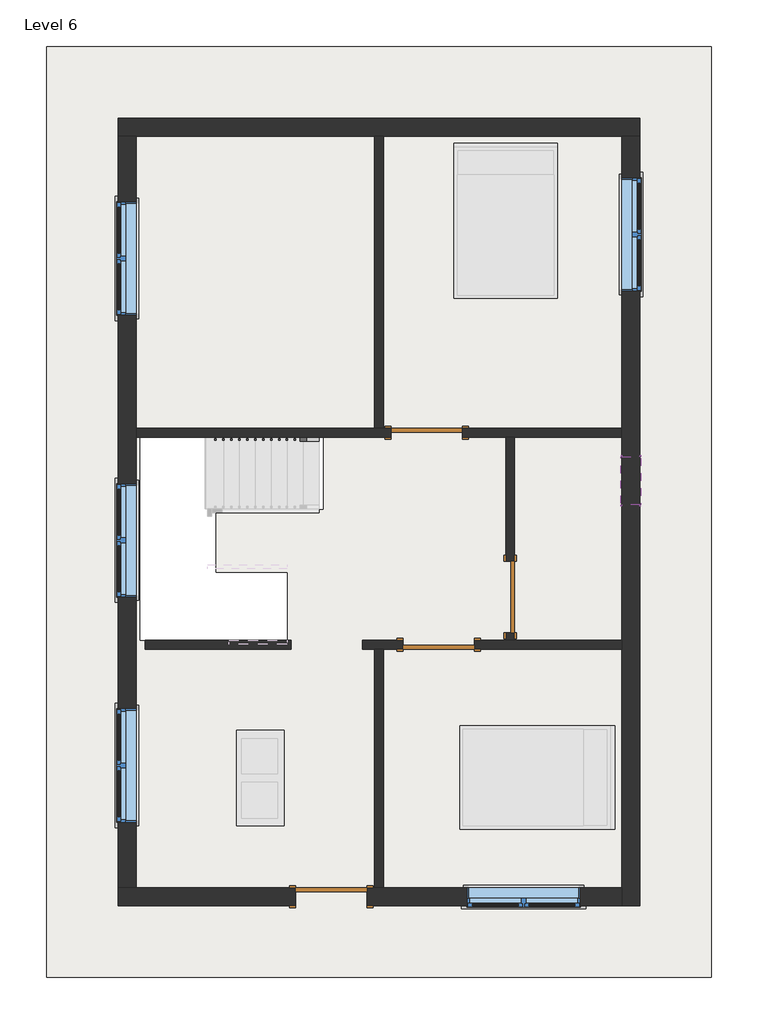
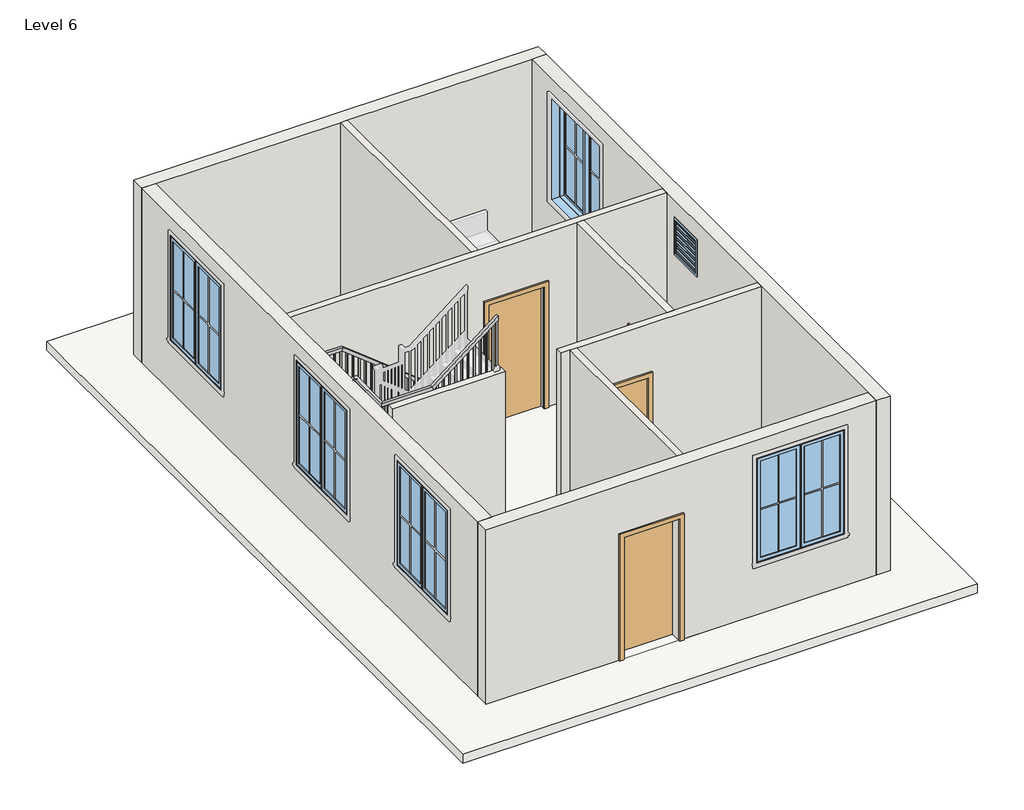
# One storey, part 1 of 2: 10 walls, 6 windows, 4 doors, 1 railing, 1 roof, 1 slab.
"""IFC4 building model written with IfcOpenShell, lengths in millimetres."""

from ifc_helpers import new_model, si_unit, frame, origin, place, context, project, spatial, polyline, outline, extrude, faceted_brep, transform, mapped, element, save
from components import door_e5f9f3c4, door_0ca8825f, window_9ac97e1a, window_f2d8fef0

model = new_model("IFC4")

# Units and contexts
model_context = context("Model", 3, world=origin())
ifc_project = project(units=[si_unit("LENGTHUNIT", "METRE", prefix="MILLI")], contexts=[model_context])

# Site, building, storey
site = spatial("IfcSite", under=ifc_project)
building = spatial("IfcBuilding", under=site)
storey = spatial("IfcBuildingStorey", under=building, Name="Level 6", Elevation=12801.6)

# Doors
placement = place(None, origin())
door_shape = door_e5f9f3c4(model_context)
element("IfcDoor", 1, ObjectType="Single-Flush : 36\" x 84\"", at=placement, inside=storey, context=model_context, shape_type="MappedRepresentation", body=[
    mapped(door_shape, transform((-2225.1840247, 979.1819954, 12801.6), x_axis=(1.0, 0.0, 0.0), y_axis=(0.0, 1.0, 0.0), z_axis=(0.0, 0.0, 1.0))),
])
element("IfcDoor", 2, ObjectType="Single-Flush : 36\" x 84\"", at=placement, inside=storey, context=model_context, shape_type="MappedRepresentation", body=[
    mapped(door_shape, transform((-1158.3840247, -1116.3180046, 12801.6), x_axis=(0.0, -1.0, 0.0), y_axis=(1.0, 0.0, 0.0), z_axis=(0.0, 0.0, 1.0))),
])
element("IfcDoor", 3, ObjectType="Single-Flush : 36\" x 84\"", at=placement, inside=storey, context=model_context, shape_type="MappedRepresentation", body=[
    mapped(door_shape, transform((-2072.7840247, -1725.9180046, 12801.6), x_axis=(-1.0, 0.0, 0.0), y_axis=(0.0, -1.0, 0.0), z_axis=(0.0, 0.0, 1.0))),
])
door_2_shape = door_0ca8825f(model_context)
element("IfcDoor", 4, ObjectType="Single-Flush : 36\" x 84\"", at=placement, inside=storey, context=model_context, shape_type="MappedRepresentation", body=[
    mapped(door_2_shape, transform((-3444.3840247, -4945.3680046, 12801.6), x_axis=(1.0, 0.0, 0.0), y_axis=(0.0, 1.0, 0.0), z_axis=(0.0, 0.0, 1.0))),
])

# Railing
element("IfcRailing", 5, ObjectType="Handrail - Rectangular", at=placement, inside=storey, context=model_context, shape_type="SolidModel", body=[
    faceted_brep([(-3603.1340247, 871.2319954, 13876.4210526), (-3603.1340247, 871.2319954, 13811.6980109), (-3603.1340247, 922.0319954, 13811.6980109), (-3603.1340247, 922.0319954, 13876.4210526), (-5097.5006913, 871.2319954, 15056.1842105), (-5115.1365442, 871.2319954, 15005.3842105), (-5115.1365442, 922.0319954, 15005.3842105), (-5097.5006913, 922.0319954, 15056.1842105), (-5889.1340247, 871.2319954, 15056.1842105), (-5889.1340247, 871.2319954, 15005.3842105), (-5939.9340247, 922.0319954, 15005.3842105), (-5939.9340247, 922.0319954, 15056.1842105), (-5889.1340247, 130.6632454, 15056.1842105), (-5889.1340247, 112.1228815, 15005.3842105), (-5939.9340247, 112.1228815, 15005.3842105), (-5939.9340247, 130.6632454, 15056.1842105), (-5889.1340247, -877.3992546, 15905.0789474), (-5889.1340247, -895.9396185, 15854.2789474), (-5939.9340247, -895.9396185, 15854.2789474), (-5939.9340247, -877.3992546, 15905.0789474), (-5889.1340247, -1617.9680046, 15905.0789474), (-5889.1340247, -1617.9680046, 15854.2789474), (-5939.9340247, -1668.7680046, 15854.2789474), (-5939.9340247, -1668.7680046, 15905.0789474), (-5097.5006913, -1617.9680046, 15905.0789474), (-5079.8648385, -1617.9680046, 15854.2789474), (-5079.8648385, -1668.7680046, 15854.2789474), (-5097.5006913, -1668.7680046, 15905.0789474), (-4009.5340247, -1617.9680046, 16764.0), (-4009.5340247, -1668.7680046, 16764.0), (-4009.5340247, -1668.7680046, 16699.2769583), (-4009.5340247, -1617.9680046, 16699.2769583)], [[[0, 1, 2, 3]], [[1, 0, 4, 5]], [[2, 1, 5, 6]], [[3, 2, 6, 7]], [[0, 3, 7, 4]], [[5, 4, 8, 9]], [[6, 5, 9, 10]], [[7, 6, 10, 11]], [[4, 7, 11, 8]], [[9, 8, 12, 13]], [[10, 9, 13, 14]], [[11, 10, 14, 15]], [[8, 11, 15, 12]], [[13, 12, 16, 17]], [[14, 13, 17, 18]], [[15, 14, 18, 19]], [[12, 15, 19, 16]], [[17, 16, 20, 21]], [[18, 17, 21, 22]], [[19, 18, 22, 23]], [[16, 19, 23, 20]], [[21, 20, 24, 25]], [[22, 21, 25, 26]], [[23, 22, 26, 27]], [[20, 23, 27, 24]], [[28, 29, 30, 31]], [[25, 24, 28, 31]], [[26, 25, 31, 30]], [[27, 26, 30, 29]], [[24, 27, 29, 28]]]),
    extrude(outline(polyline([(16646.6388004, -4076.2090247), (16631.5993267, -4095.2590247), (15689.1789474, -4095.2590247), (15689.1789474, -4076.2090247), (16646.6388004, -4076.2090247)])), frame((0.0, -1652.8930046, 0.0), z_axis=(0.0, 1.0, 0.0), x_axis=(0.0, 0.0, 1.0)), (0.0, 0.0, 1.0), 19.05),
    extrude(outline(polyline([(16566.428274, -4177.8090247), (16551.3888004, -4196.8590247), (15689.1789474, -4196.8590247), (15689.1789474, -4177.8090247), (16566.428274, -4177.8090247)])), frame((0.0, -1652.8930046, 0.0), z_axis=(0.0, 1.0, 0.0), x_axis=(0.0, 0.0, 1.0)), (0.0, 0.0, 1.0), 19.05),
    extrude(outline(polyline([(16486.2177477, -4279.4090247), (16471.178274, -4298.4590247), (15528.7578947, -4298.4590247), (15528.7578947, -4279.4090247), (16486.2177477, -4279.4090247)])), frame((0.0, -1652.8930046, 0.0), z_axis=(0.0, 1.0, 0.0), x_axis=(0.0, 0.0, 1.0)), (0.0, 0.0, 1.0), 19.05),
    extrude(outline(polyline([(16406.0072214, -4381.0090247), (16390.9677477, -4400.0590247), (15528.7578947, -4400.0590247), (15528.7578947, -4381.0090247), (16406.0072214, -4381.0090247)])), frame((0.0, -1652.8930046, 0.0), z_axis=(0.0, 1.0, 0.0), x_axis=(0.0, 0.0, 1.0)), (0.0, 0.0, 1.0), 19.05),
    extrude(outline(polyline([(16325.7966951, -4482.6090247), (16310.7572214, -4501.6590247), (15368.3368421, -4501.6590247), (15368.3368421, -4482.6090247), (16325.7966951, -4482.6090247)])), frame((0.0, -1652.8930046, 0.0), z_axis=(0.0, 1.0, 0.0), x_axis=(0.0, 0.0, 1.0)), (0.0, 0.0, 1.0), 19.05),
    extrude(outline(polyline([(16245.5861688, -4584.2090247), (16230.5466951, -4603.2590247), (15368.3368421, -4603.2590247), (15368.3368421, -4584.2090247), (16245.5861688, -4584.2090247)])), frame((0.0, -1652.8930046, 0.0), z_axis=(0.0, 1.0, 0.0), x_axis=(0.0, 0.0, 1.0)), (0.0, 0.0, 1.0), 19.05),
    extrude(outline(polyline([(16165.3756425, -4685.8090247), (16150.3361688, -4704.8590247), (15207.9157895, -4704.8590247), (15207.9157895, -4685.8090247), (16165.3756425, -4685.8090247)])), frame((0.0, -1652.8930046, 0.0), z_axis=(0.0, 1.0, 0.0), x_axis=(0.0, 0.0, 1.0)), (0.0, 0.0, 1.0), 19.05),
    extrude(outline(polyline([(16085.1651161, -4787.4090247), (16070.1256425, -4806.4590247), (15207.9157895, -4806.4590247), (15207.9157895, -4787.4090247), (16085.1651161, -4787.4090247)])), frame((0.0, -1652.8930046, 0.0), z_axis=(0.0, 1.0, 0.0), x_axis=(0.0, 0.0, 1.0)), (0.0, 0.0, 1.0), 19.05),
    extrude(outline(polyline([(16004.9545898, -4889.0090247), (15989.9151161, -4908.0590247), (15047.4947368, -4908.0590247), (15047.4947368, -4889.0090247), (16004.9545898, -4889.0090247)])), frame((0.0, -1652.8930046, 0.0), z_axis=(0.0, 1.0, 0.0), x_axis=(0.0, 0.0, 1.0)), (0.0, 0.0, 1.0), 19.05),
    extrude(outline(polyline([(15924.7440635, -4990.6090247), (15909.7045898, -5009.6590247), (15047.4947368, -5009.6590247), (15047.4947368, -4990.6090247), (15924.7440635, -4990.6090247)])), frame((0.0, -1652.8930046, 0.0), z_axis=(0.0, 1.0, 0.0), x_axis=(0.0, 0.0, 1.0)), (0.0, 0.0, 1.0), 19.05),
    extrude(outline(polyline([(-5111.2590247, -1652.8930046), (-5111.2590247, -1633.8430046), (-5092.2090247, -1633.8430046), (-5092.2090247, -1652.8930046), (-5111.2590247, -1652.8930046)])), frame((0.0, 0.0, 14887.0736842), z_axis=(0.0, 0.0, 1.0), x_axis=(1.0, 0.0, 0.0)), (0.0, 0.0, 1.0), 967.2052632),
    extrude(outline(polyline([(-5212.8590247, -1652.8930046), (-5212.8590247, -1633.8430046), (-5193.8090247, -1633.8430046), (-5193.8090247, -1652.8930046), (-5212.8590247, -1652.8930046)])), frame((0.0, 0.0, 14887.0736842), z_axis=(0.0, 0.0, 1.0), x_axis=(1.0, 0.0, 0.0)), (0.0, 0.0, 1.0), 967.2052632),
    extrude(outline(polyline([(-5314.4590247, -1652.8930046), (-5314.4590247, -1633.8430046), (-5295.4090247, -1633.8430046), (-5295.4090247, -1652.8930046), (-5314.4590247, -1652.8930046)])), frame((0.0, 0.0, 14887.0736842), z_axis=(0.0, 0.0, 1.0), x_axis=(1.0, 0.0, 0.0)), (0.0, 0.0, 1.0), 967.2052632),
    extrude(outline(polyline([(-5416.0590247, -1652.8930046), (-5416.0590247, -1633.8430046), (-5397.0090247, -1633.8430046), (-5397.0090247, -1652.8930046), (-5416.0590247, -1652.8930046)])), frame((0.0, 0.0, 14887.0736842), z_axis=(0.0, 0.0, 1.0), x_axis=(1.0, 0.0, 0.0)), (0.0, 0.0, 1.0), 967.2052632),
    extrude(outline(polyline([(-5517.6590247, -1652.8930046), (-5517.6590247, -1633.8430046), (-5498.6090247, -1633.8430046), (-5498.6090247, -1652.8930046), (-5517.6590247, -1652.8930046)])), frame((0.0, 0.0, 14887.0736842), z_axis=(0.0, 0.0, 1.0), x_axis=(1.0, 0.0, 0.0)), (0.0, 0.0, 1.0), 967.2052632),
    extrude(outline(polyline([(-5619.2590247, -1652.8930046), (-5619.2590247, -1633.8430046), (-5600.2090247, -1633.8430046), (-5600.2090247, -1652.8930046), (-5619.2590247, -1652.8930046)])), frame((0.0, 0.0, 14887.0736842), z_axis=(0.0, 0.0, 1.0), x_axis=(1.0, 0.0, 0.0)), (0.0, 0.0, 1.0), 967.2052632),
    extrude(outline(polyline([(-5720.8590247, -1652.8930046), (-5720.8590247, -1633.8430046), (-5701.8090247, -1633.8430046), (-5701.8090247, -1652.8930046), (-5720.8590247, -1652.8930046)])), frame((0.0, 0.0, 14887.0736842), z_axis=(0.0, 0.0, 1.0), x_axis=(1.0, 0.0, 0.0)), (0.0, 0.0, 1.0), 967.2052632),
    extrude(outline(polyline([(-5822.4590247, -1652.8930046), (-5822.4590247, -1633.8430046), (-5803.4090247, -1633.8430046), (-5803.4090247, -1652.8930046), (-5822.4590247, -1652.8930046)])), frame((0.0, 0.0, 14887.0736842), z_axis=(0.0, 0.0, 1.0), x_axis=(1.0, 0.0, 0.0)), (0.0, 0.0, 1.0), 967.2052632),
    extrude(outline(polyline([(-5924.0590247, -1532.2430046), (-5905.0090247, -1532.2430046), (-5905.0090247, -1551.2930046), (-5924.0590247, -1551.2930046), (-5924.0590247, -1532.2430046)])), frame((0.0, 0.0, 14887.0736842), z_axis=(0.0, 0.0, 1.0), x_axis=(1.0, 0.0, 0.0)), (0.0, 0.0, 1.0), 967.2052632),
    extrude(outline(polyline([(-5924.0590247, -1430.6430046), (-5905.0090247, -1430.6430046), (-5905.0090247, -1449.6930046), (-5924.0590247, -1449.6930046), (-5924.0590247, -1430.6430046)])), frame((0.0, 0.0, 14887.0736842), z_axis=(0.0, 0.0, 1.0), x_axis=(1.0, 0.0, 0.0)), (0.0, 0.0, 1.0), 967.2052632),
    extrude(outline(polyline([(-5924.0590247, -1329.0430046), (-5905.0090247, -1329.0430046), (-5905.0090247, -1348.0930046), (-5924.0590247, -1348.0930046), (-5924.0590247, -1329.0430046)])), frame((0.0, 0.0, 14887.0736842), z_axis=(0.0, 0.0, 1.0), x_axis=(1.0, 0.0, 0.0)), (0.0, 0.0, 1.0), 967.2052632),
    extrude(outline(polyline([(-5924.0590247, -1227.4430046), (-5905.0090247, -1227.4430046), (-5905.0090247, -1246.4930046), (-5924.0590247, -1246.4930046), (-5924.0590247, -1227.4430046)])), frame((0.0, 0.0, 14887.0736842), z_axis=(0.0, 0.0, 1.0), x_axis=(1.0, 0.0, 0.0)), (0.0, 0.0, 1.0), 967.2052632),
    extrude(outline(polyline([(-5924.0590247, -1125.8430046), (-5905.0090247, -1125.8430046), (-5905.0090247, -1144.8930046), (-5924.0590247, -1144.8930046), (-5924.0590247, -1125.8430046)])), frame((0.0, 0.0, 14887.0736842), z_axis=(0.0, 0.0, 1.0), x_axis=(1.0, 0.0, 0.0)), (0.0, 0.0, 1.0), 967.2052632),
    extrude(outline(polyline([(-5924.0590247, -1024.2430046), (-5905.0090247, -1024.2430046), (-5905.0090247, -1043.2930046), (-5924.0590247, -1043.2930046), (-5924.0590247, -1024.2430046)])), frame((0.0, 0.0, 14887.0736842), z_axis=(0.0, 0.0, 1.0), x_axis=(1.0, 0.0, 0.0)), (0.0, 0.0, 1.0), 967.2052632),
    extrude(outline(polyline([(-5924.0590247, -922.6430046), (-5905.0090247, -922.6430046), (-5905.0090247, -941.6930046), (-5924.0590247, -941.6930046), (-5924.0590247, -922.6430046)])), frame((0.0, 0.0, 14887.0736842), z_axis=(0.0, 0.0, 1.0), x_axis=(1.0, 0.0, 0.0)), (0.0, 0.0, 1.0), 967.2052632),
    extrude(outline(polyline([(-840.0930046, 15807.2502199), (-821.0430046, 15791.2081146), (-821.0430046, 14887.0736842), (-840.0930046, 14887.0736842), (-840.0930046, 15807.2502199)])), frame((-5924.0590247, 0.0, 0.0), z_axis=(1.0, 0.0, 0.0), x_axis=(0.0, 1.0, 0.0)), (0.0, 0.0, 1.0), 19.05),
    extrude(outline(polyline([(-738.4930046, 15721.6923251), (-719.4430046, 15705.6502199), (-719.4430046, 14726.6526316), (-738.4930046, 14726.6526316), (-738.4930046, 15721.6923251)])), frame((-5924.0590247, 0.0, 0.0), z_axis=(1.0, 0.0, 0.0), x_axis=(0.0, 1.0, 0.0)), (0.0, 0.0, 1.0), 19.05),
    extrude(outline(polyline([(-636.8930046, 15636.1344304), (-617.8430046, 15620.0923251), (-617.8430046, 14726.6526316), (-636.8930046, 14726.6526316), (-636.8930046, 15636.1344304)])), frame((-5924.0590247, 0.0, 0.0), z_axis=(1.0, 0.0, 0.0), x_axis=(0.0, 1.0, 0.0)), (0.0, 0.0, 1.0), 19.05),
    extrude(outline(polyline([(-535.2930046, 15550.5765357), (-516.2430046, 15534.5344304), (-516.2430046, 14566.2315789), (-535.2930046, 14566.2315789), (-535.2930046, 15550.5765357)])), frame((-5924.0590247, 0.0, 0.0), z_axis=(1.0, 0.0, 0.0), x_axis=(0.0, 1.0, 0.0)), (0.0, 0.0, 1.0), 19.05),
    extrude(outline(polyline([(-433.6930046, 15465.0186409), (-414.6430046, 15448.9765357), (-414.6430046, 14566.2315789), (-433.6930046, 14566.2315789), (-433.6930046, 15465.0186409)])), frame((-5924.0590247, 0.0, 0.0), z_axis=(1.0, 0.0, 0.0), x_axis=(0.0, 1.0, 0.0)), (0.0, 0.0, 1.0), 19.05),
    extrude(outline(polyline([(-332.0930046, 15379.4607462), (-313.0430046, 15363.4186409), (-313.0430046, 14405.8105263), (-332.0930046, 14405.8105263), (-332.0930046, 15379.4607462)])), frame((-5924.0590247, 0.0, 0.0), z_axis=(1.0, 0.0, 0.0), x_axis=(0.0, 1.0, 0.0)), (0.0, 0.0, 1.0), 19.05),
    extrude(outline(polyline([(-230.4930046, 15293.9028514), (-211.4430046, 15277.8607462), (-211.4430046, 14405.8105263), (-230.4930046, 14405.8105263), (-230.4930046, 15293.9028514)])), frame((-5924.0590247, 0.0, 0.0), z_axis=(1.0, 0.0, 0.0), x_axis=(0.0, 1.0, 0.0)), (0.0, 0.0, 1.0), 19.05),
    extrude(outline(polyline([(-128.8930046, 15208.3449567), (-109.8430046, 15192.3028514), (-109.8430046, 14245.3894737), (-128.8930046, 14245.3894737), (-128.8930046, 15208.3449567)])), frame((-5924.0590247, 0.0, 0.0), z_axis=(1.0, 0.0, 0.0), x_axis=(0.0, 1.0, 0.0)), (0.0, 0.0, 1.0), 19.05),
    extrude(outline(polyline([(-27.2930046, 15122.787062), (-8.2430046, 15106.7449567), (-8.2430046, 14245.3894737), (-27.2930046, 14245.3894737), (-27.2930046, 15122.787062)])), frame((-5924.0590247, 0.0, 0.0), z_axis=(1.0, 0.0, 0.0), x_axis=(0.0, 1.0, 0.0)), (0.0, 0.0, 1.0), 19.05),
    extrude(outline(polyline([(74.3069954, 15037.2291672), (93.3569954, 15021.187062), (93.3569954, 14084.9684211), (74.3069954, 14084.9684211), (74.3069954, 15037.2291672)])), frame((-5924.0590247, 0.0, 0.0), z_axis=(1.0, 0.0, 0.0), x_axis=(0.0, 1.0, 0.0)), (0.0, 0.0, 1.0), 19.05),
    extrude(outline(polyline([(-5924.0590247, 194.9569954), (-5905.0090247, 194.9569954), (-5905.0090247, 175.9069954), (-5924.0590247, 175.9069954), (-5924.0590247, 194.9569954)])), frame((0.0, 0.0, 14084.9684211), z_axis=(0.0, 0.0, 1.0), x_axis=(1.0, 0.0, 0.0)), (0.0, 0.0, 1.0), 920.4157895),
    extrude(outline(polyline([(-5924.0590247, 296.5569954), (-5905.0090247, 296.5569954), (-5905.0090247, 277.5069954), (-5924.0590247, 277.5069954), (-5924.0590247, 296.5569954)])), frame((0.0, 0.0, 14084.9684211), z_axis=(0.0, 0.0, 1.0), x_axis=(1.0, 0.0, 0.0)), (0.0, 0.0, 1.0), 920.4157895),
    extrude(outline(polyline([(-5924.0590247, 398.1569954), (-5905.0090247, 398.1569954), (-5905.0090247, 379.1069954), (-5924.0590247, 379.1069954), (-5924.0590247, 398.1569954)])), frame((0.0, 0.0, 14084.9684211), z_axis=(0.0, 0.0, 1.0), x_axis=(1.0, 0.0, 0.0)), (0.0, 0.0, 1.0), 920.4157895),
    extrude(outline(polyline([(-5924.0590247, 499.7569954), (-5905.0090247, 499.7569954), (-5905.0090247, 480.7069954), (-5924.0590247, 480.7069954), (-5924.0590247, 499.7569954)])), frame((0.0, 0.0, 14084.9684211), z_axis=(0.0, 0.0, 1.0), x_axis=(1.0, 0.0, 0.0)), (0.0, 0.0, 1.0), 920.4157895),
    extrude(outline(polyline([(-5924.0590247, 601.3569954), (-5905.0090247, 601.3569954), (-5905.0090247, 582.3069954), (-5924.0590247, 582.3069954), (-5924.0590247, 601.3569954)])), frame((0.0, 0.0, 14084.9684211), z_axis=(0.0, 0.0, 1.0), x_axis=(1.0, 0.0, 0.0)), (0.0, 0.0, 1.0), 920.4157895),
    extrude(outline(polyline([(-5924.0590247, 702.9569954), (-5905.0090247, 702.9569954), (-5905.0090247, 683.9069954), (-5924.0590247, 683.9069954), (-5924.0590247, 702.9569954)])), frame((0.0, 0.0, 14084.9684211), z_axis=(0.0, 0.0, 1.0), x_axis=(1.0, 0.0, 0.0)), (0.0, 0.0, 1.0), 920.4157895),
    extrude(outline(polyline([(-5924.0590247, 804.5569954), (-5905.0090247, 804.5569954), (-5905.0090247, 785.5069954), (-5924.0590247, 785.5069954), (-5924.0590247, 804.5569954)])), frame((0.0, 0.0, 14084.9684211), z_axis=(0.0, 0.0, 1.0), x_axis=(1.0, 0.0, 0.0)), (0.0, 0.0, 1.0), 920.4157895),
    extrude(outline(polyline([(-5828.8090247, 906.1569954), (-5828.8090247, 887.1069954), (-5847.8590247, 887.1069954), (-5847.8590247, 906.1569954), (-5828.8090247, 906.1569954)])), frame((0.0, 0.0, 14084.9684211), z_axis=(0.0, 0.0, 1.0), x_axis=(1.0, 0.0, 0.0)), (0.0, 0.0, 1.0), 920.4157895),
    extrude(outline(polyline([(-5727.2090247, 906.1569954), (-5727.2090247, 887.1069954), (-5746.2590247, 887.1069954), (-5746.2590247, 906.1569954), (-5727.2090247, 906.1569954)])), frame((0.0, 0.0, 14084.9684211), z_axis=(0.0, 0.0, 1.0), x_axis=(1.0, 0.0, 0.0)), (0.0, 0.0, 1.0), 920.4157895),
    extrude(outline(polyline([(-5625.6090247, 906.1569954), (-5625.6090247, 887.1069954), (-5644.6590247, 887.1069954), (-5644.6590247, 906.1569954), (-5625.6090247, 906.1569954)])), frame((0.0, 0.0, 14084.9684211), z_axis=(0.0, 0.0, 1.0), x_axis=(1.0, 0.0, 0.0)), (0.0, 0.0, 1.0), 920.4157895),
    extrude(outline(polyline([(-5524.0090247, 906.1569954), (-5524.0090247, 887.1069954), (-5543.0590247, 887.1069954), (-5543.0590247, 906.1569954), (-5524.0090247, 906.1569954)])), frame((0.0, 0.0, 14084.9684211), z_axis=(0.0, 0.0, 1.0), x_axis=(1.0, 0.0, 0.0)), (0.0, 0.0, 1.0), 920.4157895),
    extrude(outline(polyline([(-5422.4090247, 906.1569954), (-5422.4090247, 887.1069954), (-5441.4590247, 887.1069954), (-5441.4590247, 906.1569954), (-5422.4090247, 906.1569954)])), frame((0.0, 0.0, 14084.9684211), z_axis=(0.0, 0.0, 1.0), x_axis=(1.0, 0.0, 0.0)), (0.0, 0.0, 1.0), 920.4157895),
    extrude(outline(polyline([(-5320.8090247, 906.1569954), (-5320.8090247, 887.1069954), (-5339.8590247, 887.1069954), (-5339.8590247, 906.1569954), (-5320.8090247, 906.1569954)])), frame((0.0, 0.0, 14084.9684211), z_axis=(0.0, 0.0, 1.0), x_axis=(1.0, 0.0, 0.0)), (0.0, 0.0, 1.0), 920.4157895),
    extrude(outline(polyline([(-5219.2090247, 906.1569954), (-5219.2090247, 887.1069954), (-5238.2590247, 887.1069954), (-5238.2590247, 906.1569954), (-5219.2090247, 906.1569954)])), frame((0.0, 0.0, 14084.9684211), z_axis=(0.0, 0.0, 1.0), x_axis=(1.0, 0.0, 0.0)), (0.0, 0.0, 1.0), 920.4157895),
    extrude(outline(polyline([(-5117.6090247, 906.1569954), (-5117.6090247, 887.1069954), (-5136.6590247, 887.1069954), (-5136.6590247, 906.1569954), (-5117.6090247, 906.1569954)])), frame((0.0, 0.0, 14084.9684211), z_axis=(0.0, 0.0, 1.0), x_axis=(1.0, 0.0, 0.0)), (0.0, 0.0, 1.0), 920.4157895),
    extrude(outline(polyline([(14927.1256425, -5016.0090247), (14942.1651161, -5035.0590247), (14084.9684211, -5035.0590247), (14084.9684211, -5016.0090247), (14927.1256425, -5016.0090247)])), frame((0.0, 887.1069954, 0.0), z_axis=(0.0, 1.0, 0.0), x_axis=(0.0, 0.0, 1.0)), (0.0, 0.0, 1.0), 19.05),
    extrude(outline(polyline([(14846.9151161, -4914.4090247), (14861.9545898, -4933.4590247), (13924.5473684, -4933.4590247), (13924.5473684, -4914.4090247), (14846.9151161, -4914.4090247)])), frame((0.0, 887.1069954, 0.0), z_axis=(0.0, 1.0, 0.0), x_axis=(0.0, 0.0, 1.0)), (0.0, 0.0, 1.0), 19.05),
    extrude(outline(polyline([(14766.7045898, -4812.8090247), (14781.7440635, -4831.8590247), (13924.5473684, -4831.8590247), (13924.5473684, -4812.8090247), (14766.7045898, -4812.8090247)])), frame((0.0, 887.1069954, 0.0), z_axis=(0.0, 1.0, 0.0), x_axis=(0.0, 0.0, 1.0)), (0.0, 0.0, 1.0), 19.05),
    extrude(outline(polyline([(14686.4940635, -4711.2090247), (14701.5335372, -4730.2590247), (13764.1263158, -4730.2590247), (13764.1263158, -4711.2090247), (14686.4940635, -4711.2090247)])), frame((0.0, 887.1069954, 0.0), z_axis=(0.0, 1.0, 0.0), x_axis=(0.0, 0.0, 1.0)), (0.0, 0.0, 1.0), 19.05),
    extrude(outline(polyline([(14606.2835372, -4609.6090247), (14621.3230109, -4628.6590247), (13764.1263158, -4628.6590247), (13764.1263158, -4609.6090247), (14606.2835372, -4609.6090247)])), frame((0.0, 887.1069954, 0.0), z_axis=(0.0, 1.0, 0.0), x_axis=(0.0, 0.0, 1.0)), (0.0, 0.0, 1.0), 19.05),
    extrude(outline(polyline([(14526.0730109, -4508.0090247), (14541.1124846, -4527.0590247), (13603.7052632, -4527.0590247), (13603.7052632, -4508.0090247), (14526.0730109, -4508.0090247)])), frame((0.0, 887.1069954, 0.0), z_axis=(0.0, 1.0, 0.0), x_axis=(0.0, 0.0, 1.0)), (0.0, 0.0, 1.0), 19.05),
    extrude(outline(polyline([(14445.8624846, -4406.4090247), (14460.9019583, -4425.4590247), (13603.7052632, -4425.4590247), (13603.7052632, -4406.4090247), (14445.8624846, -4406.4090247)])), frame((0.0, 887.1069954, 0.0), z_axis=(0.0, 1.0, 0.0), x_axis=(0.0, 0.0, 1.0)), (0.0, 0.0, 1.0), 19.05),
    extrude(outline(polyline([(14365.6519583, -4304.8090247), (14380.6914319, -4323.8590247), (13443.2842105, -4323.8590247), (13443.2842105, -4304.8090247), (14365.6519583, -4304.8090247)])), frame((0.0, 887.1069954, 0.0), z_axis=(0.0, 1.0, 0.0), x_axis=(0.0, 0.0, 1.0)), (0.0, 0.0, 1.0), 19.05),
    extrude(outline(polyline([(14285.4414319, -4203.2090247), (14300.4809056, -4222.2590247), (13443.2842105, -4222.2590247), (13443.2842105, -4203.2090247), (14285.4414319, -4203.2090247)])), frame((0.0, 887.1069954, 0.0), z_axis=(0.0, 1.0, 0.0), x_axis=(0.0, 0.0, 1.0)), (0.0, 0.0, 1.0), 19.05),
    extrude(outline(polyline([(14205.2309056, -4101.6090247), (14220.2703793, -4120.6590247), (13282.8631579, -4120.6590247), (13282.8631579, -4101.6090247), (14205.2309056, -4101.6090247)])), frame((0.0, 887.1069954, 0.0), z_axis=(0.0, 1.0, 0.0), x_axis=(0.0, 0.0, 1.0)), (0.0, 0.0, 1.0), 19.05),
    extrude(outline(polyline([(14125.0203793, -4000.0090247), (14140.059853, -4019.0590247), (13282.8631579, -4019.0590247), (13282.8631579, -4000.0090247), (14125.0203793, -4000.0090247)])), frame((0.0, 887.1069954, 0.0), z_axis=(0.0, 1.0, 0.0), x_axis=(0.0, 0.0, 1.0)), (0.0, 0.0, 1.0), 19.05),
    extrude(outline(polyline([(14044.809853, -3898.4090247), (14059.8493267, -3917.4590247), (13122.4421053, -3917.4590247), (13122.4421053, -3898.4090247), (14044.809853, -3898.4090247)])), frame((0.0, 887.1069954, 0.0), z_axis=(0.0, 1.0, 0.0), x_axis=(0.0, 0.0, 1.0)), (0.0, 0.0, 1.0), 19.05),
    extrude(outline(polyline([(13964.5993267, -3796.8090247), (13979.6388004, -3815.8590247), (13122.4421053, -3815.8590247), (13122.4421053, -3796.8090247), (13964.5993267, -3796.8090247)])), frame((0.0, 887.1069954, 0.0), z_axis=(0.0, 1.0, 0.0), x_axis=(0.0, 0.0, 1.0)), (0.0, 0.0, 1.0), 19.05),
    extrude(outline(polyline([(13884.3888004, -3695.2090247), (13899.428274, -3714.2590247), (12962.0210526, -3714.2590247), (12962.0210526, -3695.2090247), (13884.3888004, -3695.2090247)])), frame((0.0, 887.1069954, 0.0), z_axis=(0.0, 1.0, 0.0), x_axis=(0.0, 0.0, 1.0)), (0.0, 0.0, 1.0), 19.05),
    extrude(outline(polyline([(-5924.0590247, -1633.8430046), (-5905.0090247, -1633.8430046), (-5905.0090247, -1652.8930046), (-5924.0590247, -1652.8930046), (-5924.0590247, -1633.8430046)])), frame((0.0, 0.0, 14887.0736842), z_axis=(0.0, 0.0, 1.0), x_axis=(1.0, 0.0, 0.0)), (0.0, 0.0, 1.0), 967.2052632),
    extrude(outline(polyline([(-5905.0090247, 906.1569954), (-5905.0090247, 887.1069954), (-5924.0590247, 887.1069954), (-5924.0590247, 906.1569954), (-5905.0090247, 906.1569954)])), frame((0.0, 0.0, 14084.9684211), z_axis=(0.0, 0.0, 1.0), x_axis=(1.0, 0.0, 0.0)), (0.0, 0.0, 1.0), 920.4157895),
    extrude(outline(polyline([(16699.2769583, -4009.5340247), (16684.2374846, -4028.5840247), (15689.1789474, -4028.5840247), (15689.1789474, -4009.5340247), (16699.2769583, -4009.5340247)])), frame((0.0, -1652.8930046, 0.0), z_axis=(0.0, 1.0, 0.0), x_axis=(0.0, 0.0, 1.0)), (0.0, 0.0, 1.0), 19.05),
    extrude(outline(polyline([(13811.6980109, -3603.1340247), (13826.7374846, -3622.1840247), (12962.0210526, -3622.1840247), (12962.0210526, -3603.1340247), (13811.6980109, -3603.1340247)])), frame((0.0, 887.1069954, 0.0), z_axis=(0.0, 1.0, 0.0), x_axis=(0.0, 0.0, 1.0)), (0.0, 0.0, 1.0), 19.05),
])

# Roof
element("IfcRoof", 6, ObjectType="ROOF 6\"", at=placement, inside=storey, context=model_context, shape_type="SweptSolid", body=[
    extrude(outline(polyline([(-7082.9340247, 5913.1319954), (1413.3659753, 5913.1319954), (1413.3659753, -5974.0680046), (-7082.9340247, -5974.0680046), (-7082.9340247, 5913.1319954)]), holes=[polyline([(-5889.1340247, 922.0319954), (-5889.1340247, -1668.7680046), (-4009.5340247, -1668.7680046), (-4009.5340247, -805.1680046), (-4923.9340247, -805.1680046), (-4923.9340247, 7.6319954), (-3552.3340247, 7.6319954), (-3552.3340247, 922.0319954), (-5889.1340247, 922.0319954)])]), frame((0.0, 0.0, 12649.2), z_axis=(0.0, 0.0, 1.0), x_axis=(1.0, 0.0, 0.0)), (0.0, 0.0, 1.0), 152.4),
])

# Slab
element("IfcSlab", 7, ObjectType="FLOOR 6\"", at=placement, inside=storey, context=model_context, shape_type="SweptSolid", body=[
    extrude(outline(polyline([(498.9659753, 4998.7319954), (498.9659753, -5059.6680046), (-6168.5340247, -5059.6680046), (-6168.5340247, 4998.7319954), (498.9659753, 4998.7319954)]), holes=[polyline([(-5889.1340247, 922.0319954), (-5889.1340247, -1668.7680046), (-4009.5340247, -1668.7680046), (-4009.5340247, -805.1680046), (-4923.9340247, -805.1680046), (-4923.9340247, 7.6319954), (-3552.3340247, 7.6319954), (-3552.3340247, 922.0319954), (-5889.1340247, 922.0319954)])]), frame((0.0, 0.0, 12649.2), z_axis=(0.0, 0.0, 1.0), x_axis=(1.0, 0.0, 0.0)), (0.0, 0.0, 1.0), 152.4),
])

# Walls
element("IfcWall", 8, ObjectType="WALL 4.5\"", at=placement, inside=storey, context=model_context, shape_type="SweptSolid", body=[
    extrude(outline(polyline([(-2891.9340247, 1036.3319954), (-2891.9340247, 4770.1319954), (-2777.6340247, 4770.1319954), (-2777.6340247, 1036.3319954), (-2891.9340247, 1036.3319954)])), frame((0.0, 0.0, 12801.6), z_axis=(0.0, 0.0, 1.0), x_axis=(1.0, 0.0, 0.0)), (0.0, 0.0, 1.0), 3048.0),
])
element("IfcWall", 9, ObjectType="WALL 4.5\"", at=placement, inside=storey, context=model_context, shape_type="Brep", body=[
    faceted_brep([(-1767.9840247, 922.0319954, 14935.2), (-1767.9840247, 922.0319954, 12801.6), (-1215.5340247, 922.0319954, 12801.6), (-1101.2340247, 922.0319954, 12801.6), (270.3659753, 922.0319954, 12801.6), (270.3659753, 922.0319954, 15849.6), (-1101.2340247, 922.0319954, 15849.6), (-1215.5340247, 922.0319954, 15849.6), (-3552.3340247, 922.0319954, 15849.6), (-5889.1340247, 922.0319954, 15849.6), (-5939.9340247, 922.0319954, 15849.6), (-5939.9340247, 922.0319954, 12801.6), (-2682.3840247, 922.0319954, 12801.6), (-2682.3840247, 922.0319954, 14935.2), (270.3659753, 1036.3319954, 12801.6), (-1767.9840247, 1036.3319954, 12801.6), (-1767.9840247, 1036.3319954, 14935.2), (-2682.3840247, 1036.3319954, 14935.2), (-2682.3840247, 1036.3319954, 12801.6), (-2777.6340247, 1036.3319954, 12801.6), (-2891.9340247, 1036.3319954, 12801.6), (-5939.9340247, 1036.3319954, 12801.6), (-5939.9340247, 1036.3319954, 15849.6), (-2891.9340247, 1036.3319954, 15849.6), (-2777.6340247, 1036.3319954, 15849.6), (270.3659753, 1036.3319954, 15849.6)], [[[0, 1, 2, 3, 4, 5, 6, 7, 8, 9, 10, 11, 12, 13]], [[14, 15, 16, 17, 18, 19, 20, 21, 22, 23, 24, 25]], [[12, 11, 21, 20, 19, 18]], [[4, 3, 2, 1, 15, 14]], [[5, 4, 14, 25]], [[11, 10, 22, 21]], [[16, 15, 1, 0]], [[17, 16, 0, 13]], [[18, 17, 13, 12]], [[10, 9, 8, 7, 6, 5, 25, 24, 23, 22]]]),
])
element("IfcWall", 10, ObjectType="WALL 4.5\"", at=placement, inside=storey, context=model_context, shape_type="SweptSolid", body=[
    extrude(outline(polyline([(-1573.5180046, 14935.2), (-1573.5180046, 12801.6), (-1668.7680046, 12801.6), (-1668.7680046, 15849.6), (922.0319954, 15849.6), (922.0319954, 12801.6), (-659.1180046, 12801.6), (-659.1180046, 14935.2), (-1573.5180046, 14935.2)])), frame((-1215.5340247, 0.0, 0.0), z_axis=(1.0, 0.0, 0.0), x_axis=(0.0, 1.0, 0.0)), (0.0, 0.0, 1.0), 114.3),
])
element("IfcWall", 11, ObjectType="WALL 4.5\"", at=placement, inside=storey, context=model_context, shape_type="Brep", body=[
    faceted_brep([(-2529.9840247, -1668.7680046, 14935.2), (-2529.9840247, -1668.7680046, 12801.6), (-3044.3340247, -1668.7680046, 12801.6), (-3044.3340247, -1668.7680046, 15849.6), (-1215.5340247, -1668.7680046, 15849.6), (-1101.2340247, -1668.7680046, 15849.6), (270.3659753, -1668.7680046, 15849.6), (270.3659753, -1668.7680046, 12801.6), (-1101.2340247, -1668.7680046, 12801.6), (-1215.5340247, -1668.7680046, 12801.6), (-1615.5840247, -1668.7680046, 12801.6), (-1615.5840247, -1668.7680046, 14935.2), (-3044.3340247, -1783.0680046, 12801.6), (-2891.9340247, -1783.0680046, 12801.6), (-2777.6340247, -1783.0680046, 12801.6), (-2529.9840247, -1783.0680046, 12801.6), (-2529.9840247, -1783.0680046, 14935.2), (-1615.5840247, -1783.0680046, 14935.2), (-1615.5840247, -1783.0680046, 12801.6), (270.3659753, -1783.0680046, 12801.6), (270.3659753, -1783.0680046, 15849.6), (-2777.6340247, -1783.0680046, 15849.6), (-2891.9340247, -1783.0680046, 15849.6), (-3044.3340247, -1783.0680046, 15849.6)], [[[0, 1, 2, 3, 4, 5, 6, 7, 8, 9, 10, 11]], [[12, 13, 14, 15, 16, 17, 18, 19, 20, 21, 22, 23]], [[2, 1, 15, 14, 13, 12]], [[10, 9, 8, 7, 19, 18]], [[3, 2, 12, 23]], [[7, 6, 20, 19]], [[16, 15, 1, 0]], [[17, 16, 0, 11]], [[18, 17, 11, 10]], [[6, 5, 4, 3, 23, 22, 21, 20]]]),
])
element("IfcWall", 12, ObjectType="WALL 4.5\"", at=placement, inside=storey, context=model_context, shape_type="Brep", body=[
    faceted_brep([(-5825.6340247, -1783.0680046, 12801.6), (-3958.7340247, -1783.0680046, 12801.6), (-3958.7340247, -1783.0680046, 15849.6), (-5825.6340247, -1783.0680046, 15849.6), (-5825.6340247, -1668.7680046, 12801.6), (-5825.6340247, -1668.7680046, 15849.6), (-4009.5340247, -1668.7680046, 15849.6), (-3958.7340247, -1668.7680046, 15849.6), (-3958.7340247, -1668.7680046, 12801.6)], [[[0, 1, 2, 3]], [[4, 5, 6, 7, 8]], [[1, 0, 4, 8]], [[2, 1, 8, 7]], [[0, 3, 5, 4]], [[3, 2, 7, 6, 5]]]),
])
element("IfcWall", 13, ObjectType="WALL 4.5\"", at=placement, inside=storey, context=model_context, shape_type="SweptSolid", body=[
    extrude(outline(polyline([(-2891.9340247, -4831.0680046), (-2891.9340247, -1783.0680046), (-2777.6340247, -1783.0680046), (-2777.6340247, -4831.0680046), (-2891.9340247, -4831.0680046)])), frame((0.0, 0.0, 12801.6), z_axis=(0.0, 0.0, 1.0), x_axis=(1.0, 0.0, 0.0)), (0.0, 0.0, 1.0), 3048.0),
])
element("IfcWall", 14, ObjectType="WALL 9\"", at=placement, inside=storey, context=model_context, shape_type="Brep", body=[
    faceted_brep([(-6168.5340247, 4770.1319954, 12801.6), (-5939.9340247, 4770.1319954, 12801.6), (-2891.9340247, 4770.1319954, 12801.6), (-2777.6340247, 4770.1319954, 12801.6), (270.3659753, 4770.1319954, 12801.6), (498.9659753, 4770.1319954, 12801.6), (498.9659753, 4770.1319954, 15849.6), (270.3659753, 4770.1319954, 15849.6), (-2777.6340247, 4770.1319954, 15849.6), (-2891.9340247, 4770.1319954, 15849.6), (-5939.9340247, 4770.1319954, 15849.6), (-6168.5340247, 4770.1319954, 15849.6), (-6168.5340247, 4998.7319954, 12801.6), (-6168.5340247, 4998.7319954, 15849.6), (498.9659753, 4998.7319954, 15849.6), (498.9659753, 4998.7319954, 12801.6)], [[[0, 1, 2, 3, 4, 5, 6, 7, 8, 9, 10, 11]], [[12, 13, 14, 15]], [[5, 4, 3, 2, 1, 0, 12, 15]], [[6, 5, 15, 14]], [[0, 11, 13, 12]], [[11, 10, 9, 8, 7, 6, 14, 13]]]),
])
element("IfcWall", 15, ObjectType="WALL 9\"", at=placement, inside=storey, context=model_context, shape_type="Brep", body=[
    faceted_brep([(270.3659753, 4770.1319954, 12801.6), (270.3659753, 1036.3319954, 12801.6), (270.3659753, 922.0319954, 12801.6), (270.3659753, -1668.7680046, 12801.6), (270.3659753, -1783.0680046, 12801.6), (270.3659753, -4831.0680046, 12801.6), (270.3659753, -5059.6680046, 12801.6), (270.3659753, -5059.6680046, 15849.6), (270.3659753, -4831.0680046, 15849.6), (270.3659753, -1783.0680046, 15849.6), (270.3659753, -1668.7680046, 15849.6), (270.3659753, 922.0319954, 15849.6), (270.3659753, 1036.3319954, 15849.6), (270.3659753, 4770.1319954, 15849.6), (270.3659753, 2788.9319954, 15544.8), (270.3659753, 2788.9319954, 13716.0), (270.3659753, 4236.7319954, 13716.0), (270.3659753, 4236.7319954, 15544.8), (270.3659753, 64.7819954, 15544.8), (270.3659753, 64.7819954, 14935.2), (270.3659753, 674.3819954, 14935.2), (270.3659753, 674.3819954, 15544.8), (498.9659753, 4770.1319954, 12801.6), (498.9659753, 4770.1319954, 15849.6), (498.9659753, -5059.6680046, 15849.6), (498.9659753, -5059.6680046, 12801.6), (498.9659753, 2788.9319954, 15544.8), (498.9659753, 4236.7319954, 15544.8), (498.9659753, 4236.7319954, 13716.0), (498.9659753, 2788.9319954, 13716.0), (498.9659753, 64.7819954, 15544.8), (498.9659753, 674.3819954, 15544.8), (498.9659753, 674.3819954, 14935.2), (498.9659753, 64.7819954, 14935.2)], [[[0, 1, 2, 3, 4, 5, 6, 7, 8, 9, 10, 11, 12, 13], [14, 15, 16, 17], [18, 19, 20, 21]], [[22, 23, 24, 25], [26, 27, 28, 29], [30, 31, 32, 33]], [[6, 5, 4, 3, 2, 1, 0, 22, 25]], [[0, 13, 23, 22]], [[7, 6, 25, 24]], [[15, 14, 26, 29]], [[16, 15, 29, 28]], [[17, 16, 28, 27]], [[14, 17, 27, 26]], [[19, 18, 30, 33]], [[20, 19, 33, 32]], [[21, 20, 32, 31]], [[18, 21, 31, 30]], [[13, 12, 11, 10, 9, 8, 7, 24, 23]]]),
])
element("IfcWall", 16, ObjectType="WALL 9\"", at=placement, inside=storey, context=model_context, shape_type="Brep", body=[
    faceted_brep([(270.3659753, -4831.0680046, 12801.6), (-2777.6340247, -4831.0680046, 12801.6), (-2891.9340247, -4831.0680046, 12801.6), (-2987.1840247, -4831.0680046, 12801.6), (-2987.1840247, -4831.0680046, 14935.2), (-3901.5840247, -4831.0680046, 14935.2), (-3901.5840247, -4831.0680046, 12801.6), (-5939.9340247, -4831.0680046, 12801.6), (-6168.5340247, -4831.0680046, 12801.6), (-6168.5340247, -4831.0680046, 15849.6), (-5939.9340247, -4831.0680046, 15849.6), (-2891.9340247, -4831.0680046, 15849.6), (-2777.6340247, -4831.0680046, 15849.6), (270.3659753, -4831.0680046, 15849.6), (-1710.8340247, -4831.0680046, 15544.8), (-1710.8340247, -4831.0680046, 13716.0), (-263.0340247, -4831.0680046, 13716.0), (-263.0340247, -4831.0680046, 15544.8), (-2987.1840247, -5059.6680046, 14935.2), (-2987.1840247, -5059.6680046, 12801.6), (270.3659753, -5059.6680046, 12801.6), (270.3659753, -5059.6680046, 15849.6), (-6168.5340247, -5059.6680046, 15849.6), (-6168.5340247, -5059.6680046, 12801.6), (-3901.5840247, -5059.6680046, 12801.6), (-3901.5840247, -5059.6680046, 14935.2), (-1710.8340247, -5059.6680046, 15544.8), (-263.0340247, -5059.6680046, 15544.8), (-263.0340247, -5059.6680046, 13716.0), (-1710.8340247, -5059.6680046, 13716.0)], [[[0, 1, 2, 3, 4, 5, 6, 7, 8, 9, 10, 11, 12, 13], [14, 15, 16, 17]], [[18, 19, 20, 21, 22, 23, 24, 25], [26, 27, 28, 29]], [[24, 23, 8, 7, 6]], [[20, 19, 3, 2, 1, 0]], [[0, 13, 21, 20]], [[9, 8, 23, 22]], [[15, 14, 26, 29]], [[16, 15, 29, 28]], [[17, 16, 28, 27]], [[14, 17, 27, 26]], [[4, 3, 19, 18]], [[5, 4, 18, 25]], [[6, 5, 25, 24]], [[13, 12, 11, 10, 9, 22, 21]]]),
])
element("IfcWall", 17, ObjectType="WALL 9\"", at=placement, inside=storey, context=model_context, shape_type="Brep", body=[
    faceted_brep([(-5939.9340247, -4831.0680046, 12801.6), (-5939.9340247, 922.0319954, 12801.6), (-5939.9340247, 1036.3319954, 12801.6), (-5939.9340247, 4770.1319954, 12801.6), (-5939.9340247, 4770.1319954, 15849.6), (-5939.9340247, 1036.3319954, 15849.6), (-5939.9340247, 922.0319954, 15849.6), (-5939.9340247, -4831.0680046, 15849.6), (-5939.9340247, -2545.0680046, 15544.8), (-5939.9340247, -2545.0680046, 13716.0), (-5939.9340247, -3992.8680046, 13716.0), (-5939.9340247, -3992.8680046, 15544.8), (-5939.9340247, 3931.9319954, 15544.8), (-5939.9340247, 3931.9319954, 13716.0), (-5939.9340247, 2484.1319954, 13716.0), (-5939.9340247, 2484.1319954, 15544.8), (-5939.9340247, 331.4819954, 15544.8), (-5939.9340247, 331.4819954, 13716.0), (-5939.9340247, -1116.3180046, 13716.0), (-5939.9340247, -1116.3180046, 15544.8), (-6168.5340247, -4831.0680046, 12801.6), (-6168.5340247, -4831.0680046, 15849.6), (-6168.5340247, 4770.1319954, 15849.6), (-6168.5340247, 4770.1319954, 12801.6), (-6168.5340247, -2545.0680046, 15544.8), (-6168.5340247, -3992.8680046, 15544.8), (-6168.5340247, -3992.8680046, 13716.0), (-6168.5340247, -2545.0680046, 13716.0), (-6168.5340247, 3931.9319954, 15544.8), (-6168.5340247, 2484.1319954, 15544.8), (-6168.5340247, 2484.1319954, 13716.0), (-6168.5340247, 3931.9319954, 13716.0), (-6168.5340247, 331.4819954, 15544.8), (-6168.5340247, -1116.3180046, 15544.8), (-6168.5340247, -1116.3180046, 13716.0), (-6168.5340247, 331.4819954, 13716.0)], [[[0, 1, 2, 3, 4, 5, 6, 7], [8, 9, 10, 11], [12, 13, 14, 15], [16, 17, 18, 19]], [[20, 21, 22, 23], [24, 25, 26, 27], [28, 29, 30, 31], [32, 33, 34, 35]], [[3, 2, 1, 0, 20, 23]], [[0, 7, 21, 20]], [[4, 3, 23, 22]], [[9, 8, 24, 27]], [[10, 9, 27, 26]], [[11, 10, 26, 25]], [[8, 11, 25, 24]], [[13, 12, 28, 31]], [[14, 13, 31, 30]], [[15, 14, 30, 29]], [[12, 15, 29, 28]], [[17, 16, 32, 35]], [[18, 17, 35, 34]], [[19, 18, 34, 33]], [[16, 19, 33, 32]], [[7, 6, 5, 4, 22, 21]]]),
])

# Windows
window_shape = window_9ac97e1a(model_context)
element("IfcWindow", 18, ObjectType="Window-Casement-Double : 57\" x 72\"", at=placement, inside=storey, context=model_context, shape_type="MappedRepresentation", body=[
    mapped(window_shape, transform((-986.9340247, -4945.3680046, 12801.6), x_axis=(-1.0, 0.0, 0.0), y_axis=(0.0, -1.0, 0.0), z_axis=(0.0, 0.0, 1.0))),
])
element("IfcWindow", 19, ObjectType="Window-Casement-Double : 57\" x 72\"", at=placement, inside=storey, context=model_context, shape_type="MappedRepresentation", body=[
    mapped(window_shape, transform((-6054.2340247, -3268.9680046, 12801.6), x_axis=(0.0, 1.0, 0.0), y_axis=(-1.0, 0.0, 0.0), z_axis=(0.0, 0.0, 1.0))),
])
element("IfcWindow", 20, ObjectType="Window-Casement-Double : 57\" x 72\"", at=placement, inside=storey, context=model_context, shape_type="MappedRepresentation", body=[
    mapped(window_shape, transform((384.6659753, 3512.8319954, 12801.6), x_axis=(0.0, -1.0, 0.0), y_axis=(1.0, 0.0, 0.0), z_axis=(0.0, 0.0, 1.0))),
])
element("IfcWindow", 21, ObjectType="Window-Casement-Double : 57\" x 72\"", at=placement, inside=storey, context=model_context, shape_type="MappedRepresentation", body=[
    mapped(window_shape, transform((-6054.2340247, 3208.0319954, 12801.6), x_axis=(0.0, 1.0, 0.0), y_axis=(-1.0, 0.0, 0.0), z_axis=(0.0, 0.0, 1.0))),
])
element("IfcWindow", 22, ObjectType="Window-Casement-Double : 57\" x 72\"", at=placement, inside=storey, context=model_context, shape_type="MappedRepresentation", body=[
    mapped(window_shape, transform((-6054.2340247, -392.4180046, 12801.6), x_axis=(0.0, 1.0, 0.0), y_axis=(-1.0, 0.0, 0.0), z_axis=(0.0, 0.0, 1.0))),
])
window_2_shape = window_f2d8fef0(model_context)
element("IfcWindow", 23, ObjectType="Window-Louvers : 24\" x 24\"", at=placement, inside=storey, context=model_context, shape_type="MappedRepresentation", body=[
    mapped(window_2_shape, transform((378.3159753, 369.5819954, 14020.8), x_axis=(0.0, 1.0, 0.0), y_axis=(-1.0, 0.0, 0.0), z_axis=(0.0, 0.0, 1.0))),
])

save(model, "model.ifc")

# Revit data of these elements
# Type "Single-Flush : 36\" x 84\""
#   Type Mark = "1"
#   Construction Type Id = "MDOOR"
#   Assembly Code = "C1020"
#   Analytic Construction = "Metal"
#   Thickness = 0' - 2"
#   Heat Transfer Coefficient (U) = 0.651978 BTU/(h·ft²·°F)
#   Height = 7' - 0"
#   Trim Projection Ext = 0' - 1"
#   Trim Projection Int = 0' - 1"
#   Trim Width = 0' - 3"
#   Width = 3' - 0"
#   Define Thermal Properties by = 1
#   Define Thermal Properties by = 1
#   Door Material = Door - Panel
#   Frame Material = Door - Frame
#   Visual Light Transmittance = 0
#   Solar Heat Gain Coefficient = 0
#   Function = (empty or 0)
#   Wall Closure = (empty or 0)
# Type "Handrail - Rectangular"
#   Assembly Code = "C2010400"
#   built-in parameter 1008612 = 0.0416667 (stored number, unit not read)
#   built-in parameter 1008611 = 0.0416667 (stored number, unit not read)
#   built-in parameter 1008609 = 0.333333 (stored number, unit not read)
#   built-in parameter 1008604 = 0.166667 (stored number, unit not read)
#   built-in parameter 1008603 = 0.166667 (stored number, unit not read)
#   Railing Height = 3' - 0"
#   built-in parameter 1008630 = 2
#   built-in parameter 1008610 = 2
#   built-in parameter 1008618 = Baluster - Square : 3/4"
# Type "ROOF 6\""
#   Assembly Code = "B1020"
#   Layers, outside or top first: 0' - 6" no material (function 1)
# Type "FLOOR 6\""
#   Assembly Code = "B1010"
#   Function = 0
#   Layers, outside or top first: 0' - 6" no material (function 1)
# Type "WALL 4.5\""
#   Assembly Code = "B2010"
#   Layers, outside or top first: 0' - 4 1/2" no material (function 1)
# Type "WALL 9\""
#   Assembly Code = "B2010"
#   Layers, outside or top first: 0' - 9" no material (function 1)
# Type "Window-Casement-Double : 57\" x 72\""
#   Type Mark = "17"
#   Fire Rating = "0.5h"
#   Assembly Code = "B2020100"
#   Analytic Construction = "Double glazing - domestic"
#   Frame Extension [instance default] = 0' - 0 1/4"
#   Window Inset [instance default] = 0' - 0"
#   Wall Thickness [instance default] = 0' - 6"
#   Interior Wall Closure [instance default] = 0' - 2 1/4"
#   Half Width = 2' - 4 1/2"
#   Visual Light Transmittance = 0.81
#   Thermal Resistance (R) = 1.8146 (h·ft²·°F)/BTU
#   Solar Heat Gain Coefficient = 0.76
#   Rough Width = 4' - 9 1/2"
#   Rough Height = 6' - 0 1/2"
#   Height = 6' - 0"
#   Heat Transfer Coefficient (U) = 0.5511 BTU/(h·ft²·°F)
#   Exterior Wall Closure [instance default] = 0' - 1 1/4"
#   Extension Jamb [instance default] = 0' - 2 1/4"
#   Default Sill Height = 3' - 0"
#   Width = 4' - 9"
#   Define Thermal Properties by = 0
#   Muntin Visibility = yes
#   Interior Trim Visibility [instance default] = yes
#   Exterior Trim Visibility [instance default] = yes
#   Extension Jamb Visibility [instance default] = yes
#   Interior Trim Material = Wood - Stained
#   Muntin Pattern = Muntin Pattern_2x2 : Muntin Pattern_2x2
#   Interior Trim = Trim-Window-Interior-Flat : Picture Frame
#   Interior Frame Material = Wood - Stained
#   Glass Panel Material = Glass
#   Exterior Trim Material = Clad - White
#   Exterior Trim = Trim-Window-Exterior-Flat : with Sill
#   Exterior Frame Material = Clad - White
#   Wall Closure = (empty or 0)
# Type "Window-Louvers : 24\" x 24\""
#   Type Mark = "18"
#   Construction Type Id = "GSP4R"
#   Assembly Code = "B20"
#   Analytic Construction = "1/8 in Pilkington single glazing"
#   Visual Light Transmittance = 0.9
#   Thermal Resistance (R) = 1.53941 (h·ft²·°F)/BTU
#   Solar Heat Gain Coefficient = 0.78
#   Max Height = 1' - 11.74264"
#   Height = 2' - 0"
#   Heat Transfer Coefficient (U) = 0.6496 BTU/(h·ft²·°F)
#   Blade Width [instance default] = 1' - 10 1/2"
#   Blade Vertical Thickness = 0' - 0.35355"
#   Blade Thickness = 0' - 0 1/4"
#   Blade Spacing = 0' - 1 1/2"
#   Blade Height = 0' - 1.85355"
#   Blade Depth = 0' - 3"
#   Blade Angle = 45.00°
#   Default Sill Height = 3' - 0"
#   Trim Projection_Exterior = 0' - 0 1/2"
#   Trim Projection_Interior = 0' - 0 1/2"
#   Trim Width_Exterior = 0' - 1 1/2"
#   Trim Width_Interior = 0' - 1 1/2"
#   Width = 2' - 0"
#   Max Blade Count = 12
#   Define Thermal Properties by = 1
#   Blade Count = 12
#   Frame Material = Birch
#   Louver Material = Birch
#   Trim Exterior Material = Birch
#   Trim Interior Material = Birch
#   Wall Closure = (empty or 0)
# Elements 1, 2, 3, 4 (IfcDoor, "Single-Flush : 36\" x 84\"")
#   Phase Created = New Construction
#   Materials on its faces: "Door - Frame", "Door - Panel"
# Element 5 (IfcRailing, "Handrail - Rectangular")
#   Phase Created = New Construction
# Element 6 (IfcRoof, "ROOF 6\"")
#   built-in parameter 1001705 = 42 (stored number, unit not read)
#   built-in parameter 1001701 = -0.5 (stored number, unit not read)
#   built-in parameter 1001710 = 33615
#   Phase Created = New Construction
#   Materials on its faces: "Default Roof", "Oak Flooring"
# Element 7 (IfcSlab, "FLOOR 6\"")
#   Height Offset From Level = 0' - 0"
#   Phase Created = New Construction
#   Materials on its faces: "Default Floor"
# Elements 8, 9, 10, 11, 12, 13 (IfcWall, "WALL 4.5\"")
#   Top Offset = 0' - 0"
#   Base Offset = 0' - 0"
#   Unconnected Height = 10' - 0"
#   wall height = 10' - 0"
#   Phase Created = New Construction
#   Base Constraint = Level 6
#   Materials on its faces: "Default Wall"
# Elements 14, 15, 16, 17 (IfcWall, "WALL 9\"")
#   Top Offset = 0' - 0"
#   Base Offset = 0' - 0"
#   Unconnected Height = 10' - 0"
#   wall height = 10' - 0"
#   Phase Created = New Construction
#   Base Constraint = Level 6
#   Materials on its faces: "Default Wall", "Parking Stripe"
# Element 18 (IfcWindow, "Window-Casement-Double : 57\" x 72\"")
#   Mark = "25"
#   Window Inset = 0' - 0"
#   Interior Wall Closure = 0' - 2 1/4"
#   Frame Extension = 0' - 0 1/4"
#   Exterior Wall Closure = 0' - 1 1/4"
#   Interior Trim Visibility = yes
#   Exterior Trim Visibility = yes
#   Phase Created = New Construction
#   Materials on its faces: "Wood - Stained", "Glass", "Clad - White"
# Element 19 (IfcWindow, "Window-Casement-Double : 57\" x 72\"")
#   Mark = "26"
#   Window Inset = 0' - 0"
#   Interior Wall Closure = 0' - 2 1/4"
#   Frame Extension = 0' - 0 1/4"
#   Exterior Wall Closure = 0' - 1 1/4"
#   Interior Trim Visibility = yes
#   Exterior Trim Visibility = yes
#   Phase Created = New Construction
#   Materials on its faces: "Wood - Stained", "Glass", "Clad - White"
# Element 20 (IfcWindow, "Window-Casement-Double : 57\" x 72\"")
#   Mark = "27"
#   Window Inset = 0' - 0"
#   Interior Wall Closure = 0' - 2 1/4"
#   Frame Extension = 0' - 0 1/4"
#   Exterior Wall Closure = 0' - 1 1/4"
#   Interior Trim Visibility = yes
#   Exterior Trim Visibility = yes
#   Phase Created = New Construction
#   Materials on its faces: "Wood - Stained", "Glass", "Clad - White"
# Element 21 (IfcWindow, "Window-Casement-Double : 57\" x 72\"")
#   Mark = "28"
#   Window Inset = 0' - 0"
#   Interior Wall Closure = 0' - 2 1/4"
#   Frame Extension = 0' - 0 1/4"
#   Exterior Wall Closure = 0' - 1 1/4"
#   Interior Trim Visibility = yes
#   Exterior Trim Visibility = yes
#   Phase Created = New Construction
#   Materials on its faces: "Wood - Stained", "Glass", "Clad - White"
# Element 22 (IfcWindow, "Window-Casement-Double : 57\" x 72\"")
#   Mark = "29"
#   Window Inset = 0' - 0"
#   Interior Wall Closure = 0' - 2 1/4"
#   Frame Extension = 0' - 0 1/4"
#   Exterior Wall Closure = 0' - 1 1/4"
#   Interior Trim Visibility = yes
#   Exterior Trim Visibility = yes
#   Phase Created = New Construction
#   Materials on its faces: "Wood - Stained", "Glass", "Clad - White"
# Element 23 (IfcWindow, "Window-Louvers : 24\" x 24\"")
#   Mark = "30"
#   Blade Width = 1' - 10 1/2"
#   Phase Created = New Construction
#   Materials on its faces: "Birch"
# Materials
#   "Door - Panel": class "Wood", colour RGB 210 159 95, transparency 0, Cost = 0
#   "Door - Frame": colour RGB 118 70 51, transparency 0, Cost = 0
#   "Wood - Stained": class "Wood", colour RGB 224 178 126, transparency 0, Cost = 0
#   "Glass": class "Glass", colour RGB 0 128 192, transparency 0.75, Description = "Soda Lime Glass", Cost = 0
#   "Clad - White": class "Wood", colour RGB 242 242 238, transparency 0, Cost = 0
#   "Birch": class "Wood", colour RGB 224 178 126, transparency 0, Description = "Betula Alleghaniensis", Cost = 0
#   "Default Roof": colour RGB 88 101 114, transparency 0, Cost = 0
#   "Oak Flooring": class "Wood", colour RGB 216 169 114, transparency 0, Description = "Quercus Rubra", Cost = 0
#   "Default Floor": colour RGB 128 128 128, transparency 0, Cost = 0
#   "Default Wall": colour RGB 128 128 128, transparency 0, Cost = 0
#   "Parking Stripe": class "Paint", colour RGB 250 250 91, transparency 0, Cost = 0
